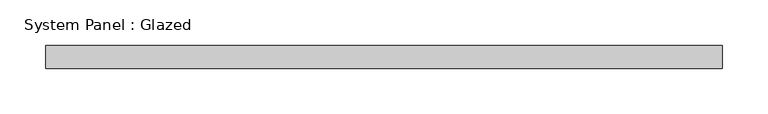
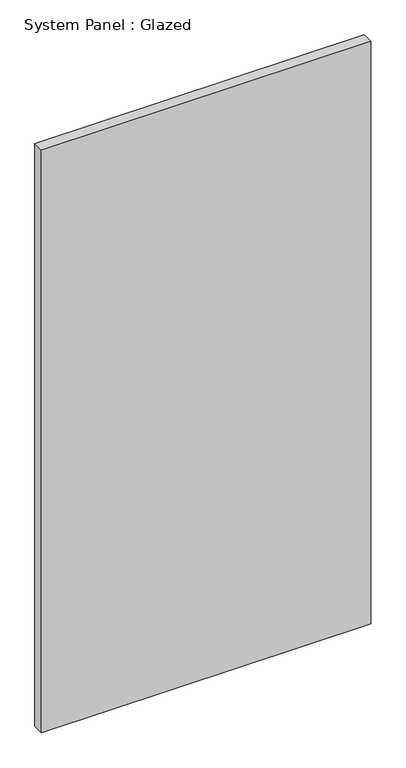
"""IFC4 building model written with IfcOpenShell, lengths in millimetres: plate geometry, System Panel : Glazed."""

from ifc_helpers import new_model, si_unit, origin, origin_with_axes, place, context, project, spatial, polyline, outline, extrude, source, transform, mapped, element, save


def system_panel_glazed_af7a4178(model_context):
    return source(origin(), model_context, "Body", "SweptSolid", [
        extrude(outline(polyline([(371.475, 19.05), (-371.475, 19.05), (-371.475, 44.45), (371.475, 44.45), (371.475, 19.05)])), origin_with_axes(), (0.0, 0.0, 1.0), 1389.4056705),
    ])


if __name__ == "__main__":
    model = new_model("IFC4")
    model_context = context("Model", 3, world=origin())
    ifc_project = project(units=[si_unit("LENGTHUNIT", "METRE", prefix="MILLI")], contexts=[model_context])
    site = spatial("IfcSite", under=ifc_project)
    building = spatial("IfcBuilding", under=site)
    placement = place(None, origin())
    system_panel_glazed_shape = system_panel_glazed_af7a4178(model_context)
    element("IfcPlate", 1, ObjectType="System Panel : Glazed", at=placement, inside=building, context=model_context, shape_type="MappedRepresentation", body=[
        mapped(system_panel_glazed_shape, transform((0.0, 0.0, 0.0), x_axis=(1.0, 0.0, 0.0), y_axis=(0.0, 1.0, 0.0), z_axis=(0.0, 0.0, 1.0))),
    ])
    save(model, "model.ifc")

# Revit data of these elements
# Type "System Panel : Glazed"
#   Construction Type Id = "GSP4R"
#   Analytic Construction = "1/8 in Pilkington single glazing"
#   Visual Light Transmittance = 0.9
#   Solar Heat Gain Coefficient = 0.86
#   Heat Transfer Coefficient (U) = 1.18115 BTU/(h·ft²·°F)
#   Define Thermal Properties by = 1
# Element 1 (IfcPlate, "System Panel : Glazed")
#   Materials on its faces: "Glass"
# Materials
#   "Glass": class "Glass", colour RGB 0 128 192, transparency 0.75, Description = "Soda Lime Glass", Cost = 0
